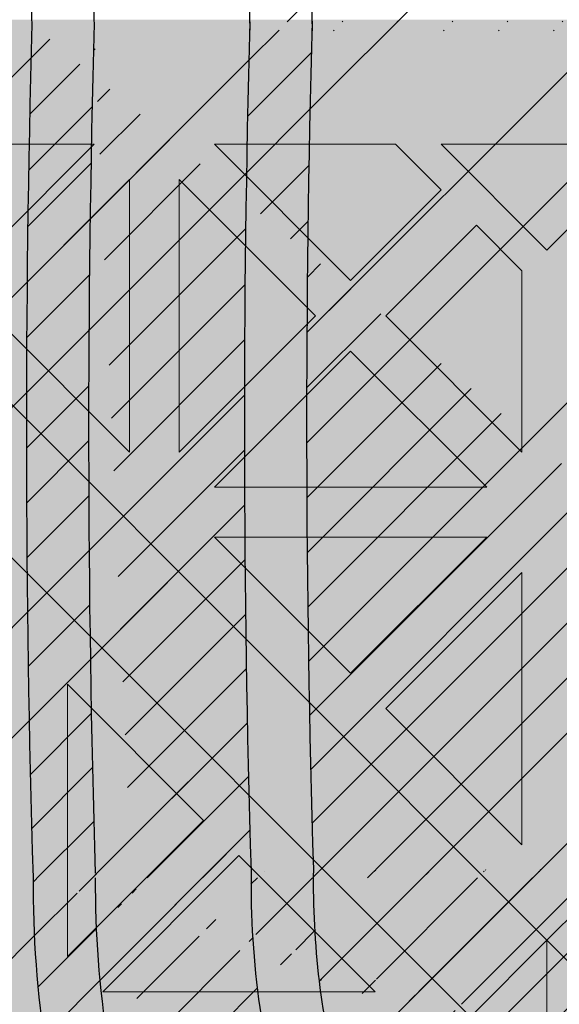
# Model space of a CAD drawing. Units: inches. Extents: x 844 to 2234, y 346 to 1084.
# Tile 54 of 93: x 1866.641 to 1869.404, y 696.327 to 701.365. Entities that reach past the tile are written whole.
import ezdxf

# ---------------------------------------------------------------- set-up
doc = ezdxf.new("R2010")
doc.units = ezdxf.units.IN
doc.header["$MEASUREMENT"] = 0
doc.layers.add('furniture', color=8, linetype='Continuous', lineweight=18)
doc.layers.add('RA-AP-01$0$INT', color=35, linetype='Continuous', lineweight=5)
doc.layers.add('RA-AP-01$0$FURN', color=3, linetype='Continuous')
doc.layers.add('RA-AP-01$0$WOOD', color=64, linetype='Continuous')

# ---------------------------------------------------------------- blocks, each defined once
blk = doc.blocks.new('A$C18D01794')
at = {"layer": 'RA-AP-01$0$INT'}
h = blk.add_hatch(color=256, dxfattribs=at)
h.paths.add_polyline_path([(4.585917135068449, -6.356712009588271), (4.555206456959269, -6.35671200958746), (4.555206456959137, -6.387422687716308), (4.874495778835233, -6.706712009592356), (4.90520645695423, -6.676001331474049)])
h.paths.add_polyline_path([(5.255206456948813, -6.387422687716306), (5.255206456948682, -6.356712009605972), (5.224495778822613, -6.356712009605161), (4.905206456953498, -6.676001331474273), (4.935917135072151, -6.706712009592924)])
h.paths.add_polyline_path([(4.935917135072559, -6.706712009592068), (4.905206456953564, -6.737422687710376), (5.255206456951813, -7.087422687708613), (5.255206456951549, -7.026001331471008)])
h.paths.add_polyline_path([(4.555206456956399, -7.026001331471013), (4.555206456956134, -7.087422687708616), (4.905206456953821, -6.737422687710943), (4.874495778835166, -6.70671200959229)])
h = blk.add_hatch(color=256, dxfattribs=at)
h.paths.add_polyline_path([(4.585917135068448, -6.356712009588273), (4.614201406330596, -6.356712009589021), (4.668846067270487, -6.411356670531338), (4.723490728212344, -6.356712009591912), (4.771774999457151, -6.35671200959319), (4.826419660396886, -6.411356670535356), (4.862780050090322, -6.374996280843536), (4.844495778842715, -6.356712009595112), (4.862780050090411, -6.356712009595595), (4.905206456960182, -6.399138416468211), (4.947632863832445, -6.356712009597838), (4.965917135079675, -6.356712009598322), (4.947632863831759, -6.374996280845421), (4.983993253523576, -6.411356670538857), (5.038637914464627, -6.356712009600247), (5.08692218571208, -6.356712009601523), (5.141566846649976, -6.411356670541852), (5.196211507589851, -6.356712009604411), (5.224495778822615, -6.356712009605161), (4.905206456953975, -6.676001331473793)])
h.paths.add_polyline_path([(4.895206456956031, -6.637717060225675), (4.895206456958921, -6.528427738347902), (4.840561796018589, -6.583072399285802)], flags=16)
h.paths.add_polyline_path([(4.915206456955638, -6.637717060226121), (4.969851117895509, -6.583072399288678), (4.915206456957609, -6.528427738348344)], flags=16)
h.paths.add_polyline_path([(4.826419660395175, -6.568930263661755), (4.881064321335613, -6.514285602723745), (4.771774999456703, -6.514285602720857)], flags=16)
h.paths.add_polyline_path([(4.983993253519558, -6.568930263665262), (5.038637914460456, -6.514285602726792), (4.929348592581548, -6.514285602724816)], flags=16)
h.paths.add_polyline_path([(4.881064321336025, -6.494285602723742), (4.826419660397532, -6.439640941782821), (4.771774999457062, -6.494285602720859)], flags=16)
h.paths.add_polyline_path([(4.929348592582019, -6.494285602724817), (5.038637914460982, -6.494285602726792), (4.983993253522945, -6.439640941786327)], flags=16)
h.paths.add_polyline_path([(4.895206456960191, -6.480143467100443), (4.895206456962115, -6.407422687715913), (4.876922185715016, -6.389138416467584), (4.840561796021581, -6.425498806159401)], flags=16)
h.paths.add_polyline_path([(4.915206456958487, -6.480143467100889), (4.969851117899527, -6.425498806162279), (4.933490728206909, -6.389138416468043), (4.9152064569598, -6.40742268771434)], flags=16)
h.paths.add_polyline_path([(4.757632863832376, -6.480143467096812), (4.812277524772842, -6.425498806158772), (4.757632863834348, -6.370854145217844)], flags=16)
h.paths.add_polyline_path([(4.737632863832376, -6.480143467096286), (4.737632863834348, -6.370854145217375), (4.682988202893906, -6.425498806155385)], flags=16)
h.paths.add_polyline_path([(5.05278005008503, -6.480143467103376), (5.052780050087917, -6.370854145224413), (4.998135389146995, -6.425498806162908)], flags=16)
h.paths.add_polyline_path([(5.072780050085024, -6.480143467103744), (5.127424711025931, -6.42549880616527), (5.072780050087916, -6.370854145224832)], flags=16)
h.paths.add_polyline_path([(4.935917135072783, -6.706712009592292), (5.255206456948811, -6.387422687716309), (5.255206456948932, -6.415706958964177), (5.200561796010279, -6.470351619902839), (5.255206456949403, -6.524996280841948), (5.25520645694961, -6.5732805520894), (5.200561796009787, -6.627925213029239), (5.236922185702417, -6.664285602721864), (5.255206456949919, -6.646001331474357), (5.255206456949998, -6.664285602721898), (5.212780050078687, -6.706712009592262), (5.25520645695036, -6.749138416463932), (5.255206456950438, -6.767422687711313), (5.236922185702424, -6.749138416463297), (5.200561796009796, -6.785498806155928), (5.255206456950753, -6.840143467096874), (5.25520645695096, -6.888427738341682), (5.200561796010322, -6.943072399282328), (5.255206456951428, -6.997717060223427), (5.255206456951547, -7.026001331471006)])
h.paths.add_polyline_path([(5.042988202883395, -6.785498806155427), (5.097632863823085, -6.840143467095101), (5.097632863822622, -6.730854145216193)], flags=16)
h.paths.add_polyline_path([(5.028846067259663, -6.771356670531693), (5.083490728198774, -6.716712009592573), (4.974201406321001, -6.716712009593042)], flags=16)
h.paths.add_polyline_path([(5.117632863823087, -6.840143467095186), (5.172277524762331, -6.785498806155926), (5.11763286382262, -6.730854145216225)], flags=16)
h.paths.add_polyline_path([(5.08349072819877, -6.696712009593886), (5.028846067259652, -6.642067348654775), (4.974201406320998, -6.696712009593438)], flags=16)
h.paths.add_polyline_path([(5.131774999446817, -6.854285602718917), (5.186419660386065, -6.799640941779662), (5.241064321325782, -6.854285602719365)], flags=17)
h.paths.add_polyline_path([(5.131774999446228, -6.716712009592374), (5.186419660386065, -6.771356670532194), (5.222780050079488, -6.734996280838764), (5.204495778832781, -6.716712009592063)], flags=16)
h.paths.add_polyline_path([(5.097632863822613, -6.682569873970264), (5.097632863823061, -6.573280552091354), (5.042988202883383, -6.627925213031044)], flags=16)
h.paths.add_polyline_path([(5.131774999446899, -6.874285602718915), (5.241064321325809, -6.874285602719364), (5.186419660386591, -6.928930263658598)], flags=17)
h.paths.add_polyline_path([(5.131774999446226, -6.696712009594078), (5.204495778830767, -6.696712009594374), (5.22278005007868, -6.67842773834687), (5.186419660386049, -6.642067348654249)], flags=16)
h.paths.add_polyline_path([(5.11763286382262, -6.682569873970225), (5.17227752476232, -6.627925213030515), (5.117632863823064, -6.573280552091267)], flags=16)
h.paths.add_polyline_path([(5.186419660386069, -6.613783077405491), (5.241064321325754, -6.559138416465795), (5.131774999446791, -6.559138416466263)], flags=16)
h.paths.add_polyline_path([(5.131774999446872, -6.539138416466263), (5.24106432132578, -6.539138416465794), (5.186419660386554, -6.484493755526573)], flags=16)
h.paths.add_polyline_path([(5.255206456951811, -7.08742268770861), (5.255206456951895, -7.106712009588038), (4.555206456956052, -7.106712009588038), (4.555206456956136, -7.087422687708617), (4.905206456953973, -6.737422687710788)])
h.paths.add_polyline_path([(4.983993253513404, -6.8444937555241), (4.92934859257295, -6.899138416462108), (5.03863791445186, -6.899138416465014)], flags=16)
h.paths.add_polyline_path([(4.969851117889988, -6.83035161990006), (4.915206456952556, -6.775706958960171), (4.915206456949648, -6.884996280837944)], flags=16)
h.paths.add_polyline_path([(4.929348592572535, -6.919138416462105), (4.983993253511019, -6.973783077403037), (5.038637914451496, -6.919138416465012)], flags=16)
h.paths.add_polyline_path([(5.052780050074912, -6.93328055208906), (4.998135389134438, -6.987925213027088), (5.052780050072919, -7.042569873968025)], flags=16)
h.paths.add_polyline_path([(5.07278005007491, -6.933280552089588), (5.072780050072918, -7.042569873968497), (5.127424711013374, -6.987925213030498)], flags=16)
h.paths.add_polyline_path([(4.89520645695295, -6.775706958959721), (4.840561796013067, -6.830351619897157), (4.895206456950961, -6.884996280837494)], flags=16)
h.paths.add_polyline_path([(4.915206456948365, -6.933280552085403), (4.915206456946434, -7.006001331471951), (4.933490728192729, -7.024285602719066), (4.969851117886972, -6.987925213026453)], flags=16)
h.paths.add_polyline_path([(4.881064321327021, -6.899138416461022), (4.82641966038902, -6.84449375552057), (4.771774999448108, -6.899138416459029)], flags=16)
h.paths.add_polyline_path([(4.895206456950073, -6.933280552084951), (4.840561796009022, -6.987925213023558), (4.876922185700835, -7.024285602716997), (4.895206456948749, -7.006001331469487)], flags=16)
h.paths.add_polyline_path([(4.983993253510392, -7.0020673486505), (4.947632863816944, -7.038427738342319), (4.965917135064043, -7.05671200959023), (5.038637914448995, -7.056712009591555)], flags=16)
h.paths.add_polyline_path([(4.881064321326543, -6.91913841646102), (4.771774999447578, -6.919138416459031), (4.826419660385607, -6.973783077399508)], flags=16)
h.paths.add_polyline_path([(4.905206456946447, -7.014285602717636), (4.862780050074785, -7.056712009588352), (4.947632863816685, -7.056712009589775)], flags=16)
h.paths.add_polyline_path([(5.14156684663679, -7.002067348654549), (5.086922185696452, -7.056712009592438), (5.196211507574223, -7.056712009594425)], flags=16)
h.paths.add_polyline_path([(4.8264196603837, -7.002067348646972), (4.771774999442643, -7.056712009585575), (4.8444957788276, -7.056712009587508), (4.862780050075511, -7.038427738340416)], flags=16)
h.paths.add_polyline_path([(4.812277524760289, -6.98792521302292), (4.757632863822258, -6.933280552082447), (4.757632863819352, -7.042569873961408)], flags=16)
h.paths.add_polyline_path([(4.73763286382226, -6.933280552082079), (4.682988202881349, -6.987925213020536), (4.737632863819352, -7.04256987396099)], flags=16)
h.paths.add_polyline_path([(4.723490728195188, -7.056712009584289), (4.668846067257299, -7.002067348643949), (4.614201406317417, -7.056712009581383)], flags=16)
h.paths.add_polyline_path([(4.597632863829262, -6.706712009592262), (4.555206456957951, -6.664285602721896), (4.555206456958029, -6.646001331474357), (4.573490728205535, -6.664285602721864), (4.609851117898167, -6.627925213029238), (4.555206456958338, -6.573280552089402), (4.555206456958546, -6.524996280841952), (4.60985111789767, -6.470351619902839), (4.555206456959015, -6.415706958964177), (4.555206456959138, -6.387422687716309), (4.874495778835167, -6.70671200959229), (4.5552064569564, -7.026001331471015), (4.555206456956523, -6.997717060223433), (4.609851117897629, -6.94307239928233), (4.555206456956988, -6.888427738341681), (4.555206456957198, -6.840143467096881), (4.609851117898153, -6.78549880615593), (4.573490728205528, -6.749138416463297), (4.555206456957507, -6.76742268771132), (4.555206456957585, -6.749138416463933)])
h.paths.add_polyline_path([(4.712780050085332, -6.730854145216195), (4.712780050084863, -6.840143467095105), (4.767424711024555, -6.785498806155427)], flags=16)
h.paths.add_polyline_path([(4.726922185709173, -6.716712009592573), (4.781566846648288, -6.771356670531693), (4.836211507586949, -6.716712009593043)], flags=16)
h.paths.add_polyline_path([(4.692780050085327, -6.730854145216225), (4.638135389145619, -6.785498806155928), (4.692780050084865, -6.840143467095185)], flags=16)
h.paths.add_polyline_path([(4.726922185709182, -6.696712009593886), (4.836211507586949, -6.696712009593436), (4.7815668466483, -6.642067348654773)], flags=16)
h.paths.add_polyline_path([(4.678637914461726, -6.71671200959237), (4.605917135075169, -6.716712009592063), (4.587632863828464, -6.734996280838766), (4.623993253521887, -6.771356670532195)], flags=16)
h.paths.add_polyline_path([(4.712780050085336, -6.68256987397026), (4.767424711024568, -6.627925213031042), (4.71278005008489, -6.573280552091352)], flags=16)
h.paths.add_polyline_path([(4.678637914461726, -6.696712009594076), (4.623993253521899, -6.642067348654247), (4.587632863829271, -6.67842773834687), (4.605917135077185, -6.696712009594376)], flags=16)
h.paths.add_polyline_path([(4.692780050085336, -6.682569873970228), (4.692780050084889, -6.573280552091267), (4.638135389145632, -6.627925213030515)], flags=16)
h.paths.add_polyline_path([(4.623993253521885, -6.799640941779662), (4.678637914461131, -6.854285602718915), (4.56934859258217, -6.854285602719365)], flags=17)
h.paths.add_polyline_path([(4.623993253521901, -6.613783077405509), (4.678637914461158, -6.559138416466263), (4.569348592582195, -6.559138416465795)], flags=16)
h.paths.add_polyline_path([(4.678637914461051, -6.874285602718915), (4.623993253521361, -6.928930263658598), (4.569348592582143, -6.874285602719364)], flags=17)
h.paths.add_polyline_path([(4.678637914461076, -6.539138416466263), (4.623993253521399, -6.484493755526573), (4.569348592582167, -6.539138416465796)], flags=16)
h = blk.add_hatch(color=256, dxfattribs=at)
h.paths.add_polyline_path([(4.781566846647504, -6.771356670530272), (4.836211507586161, -6.716712009591613), (4.726922185708388, -6.716712009591159)])
h.paths.add_polyline_path([(4.836211507586161, -6.696712009592008), (4.781566846647504, -6.642067348653354), (4.726922185708388, -6.69671200959247)])
h.paths.add_polyline_path([(4.76742471102377, -6.627925213029623), (4.712780050084083, -6.57328055208994), (4.712780050084542, -6.68256987396885)])
h.paths.add_polyline_path([(4.692780050084544, -6.682569873968819), (4.692780050084084, -6.573280552089856), (4.638135389144834, -6.627925213029111)])
h.paths.add_polyline_path([(4.678637914460932, -6.696712009592669), (4.623993253521102, -6.642067348652844), (4.587632863827676, -6.678427738346266), (4.605917135074382, -6.696712009592973)])
h.paths.add_polyline_path([(4.573490728204743, -6.664285602721736), (4.60985111789737, -6.627925213029108), (4.555206456957541, -6.573280552089279), (4.555206456957237, -6.646001331474231)])
h.paths.add_polyline_path([(4.623993253521098, -6.613783077405377), (4.67863791446035, -6.559138416466126), (4.56934859258139, -6.559138416465669)])
h.paths.add_polyline_path([(4.678637914460275, -6.539138416466126), (4.623993253520583, -6.48449375552644), (4.56934859258136, -6.539138416465672)])
h.paths.add_polyline_path([(4.609851117896854, -6.470351619902707), (4.555206456958196, -6.415706958964051), (4.555206456957738, -6.524996280841822)])
h.paths.add_polyline_path([(4.597632863828475, -6.706712009592775), (4.555206456957283, -6.664285602721582), (4.555206456956805, -6.749138416463489)])
h.paths.add_polyline_path([(4.678637914460932, -6.716712009590963), (4.605917135076396, -6.71671200959066), (4.587632863828479, -6.734996280838164), (4.623993253521104, -6.771356670530792)])
h.paths.add_polyline_path([(4.692780050084091, -6.840143467093776), (4.692780050084548, -6.730854145214809), (4.638135389144834, -6.785498806154524)])
h.paths.add_polyline_path([(4.767424711023772, -6.785498806154004), (4.712780050084545, -6.730854145214786), (4.712780050084089, -6.840143467093692)])
h.paths.add_polyline_path([(4.67863791446036, -6.854285602718778), (4.623993253521105, -6.799640941779527), (4.569348592581399, -6.854285602719237)])
h.paths.add_polyline_path([(4.609851117897371, -6.785498806155798), (4.573490728204743, -6.74913841646317), (4.555206456957237, -6.767422687710675), (4.555206456957548, -6.840143467095629)])
h.paths.add_polyline_path([(4.623993253520596, -6.928930263658465), (4.67863791446028, -6.874285602718778), (4.569348592581367, -6.874285602719238)])
h.paths.add_polyline_path([(4.609851117896867, -6.943072399282199), (4.555206456957749, -6.888427738343082), (4.55520645695821, -6.997717060220857)])
h = blk.add_hatch(color=256, dxfattribs=at)
h.paths.add_polyline_path([(4.905206456953579, -6.70671200959253), (4.905206456953751, -6.676001331474523), (4.874495778835229, -6.706712009592358)])
h.paths.add_polyline_path([(4.935917135071924, -6.706712009592703), (4.905206456953583, -6.706712009592529), (4.90520645695341, -6.737422687710532)])
h = blk.add_hatch(color=256, dxfattribs=at)
h.paths.add_polyline_path([(4.905206456953409, -6.737422687710532), (4.90520645695358, -6.706712009592529), (4.874495778835235, -6.706712009592359)])
h.paths.add_polyline_path([(4.935917135071928, -6.706712009592703), (4.905206456953754, -6.676001331474527), (4.905206456953582, -6.706712009592529)])
h = blk.add_hatch(color=256, dxfattribs=at)
h.paths.add_polyline_path([(4.895206456952951, -6.77570695895972), (4.840561796013068, -6.830351619897156), (4.895206456950958, -6.884996280837495)])
h.paths.add_polyline_path([(4.915206456949649, -6.884996280837942), (4.969851117889987, -6.830351619900054), (4.915206456952556, -6.775706958960171)])
h.paths.add_polyline_path([(5.038637914451862, -6.899138416465013), (4.983993253513403, -6.8444937555241), (4.929348592572953, -6.899138416462106)])
h.paths.add_polyline_path([(4.929348592572535, -6.919138416462105), (4.983993253511018, -6.973783077403037), (5.038637914451497, -6.919138416465012)])
h.paths.add_polyline_path([(4.915206456948366, -6.933280552085397), (4.915206456946433, -7.006001331471951), (4.93349072819273, -7.024285602719068), (4.969851117886972, -6.987925213026454)])
h.paths.add_polyline_path([(5.038637914448995, -7.056712009591553), (4.983993253510389, -7.002067348650502), (4.947632863816946, -7.038427738342318), (4.965917135064043, -7.05671200959023)])
h.paths.add_polyline_path([(5.05278005007292, -7.042569873968023), (5.05278005007491, -6.933280552089059), (4.998135389134438, -6.987925213027088)])
h.paths.add_polyline_path([(5.07278005007292, -7.042569873968496), (5.127424711013374, -6.987925213030498), (5.072780050074909, -6.933280552089588)])
h.paths.add_polyline_path([(5.141566846636789, -7.002067348654547), (5.086922185696449, -7.056712009592438), (5.196211507574223, -7.056712009594425)])
h.paths.add_polyline_path([(4.947632863816688, -7.056712009589774), (4.905206456946449, -7.014285602717634), (4.862780050074784, -7.056712009588353)])
h.paths.add_polyline_path([(4.840561796009025, -6.987925213023556), (4.876922185700834, -7.024285602716997), (4.895206456948747, -7.006001331469488), (4.895206456950075, -6.933280552084953)])
h.paths.add_polyline_path([(4.88106432132654, -6.919138416461021), (4.771774999447577, -6.919138416459031), (4.826419660385606, -6.973783077399508)])
h.paths.add_polyline_path([(4.881064321327019, -6.899138416461022), (4.826419660389019, -6.844493755520571), (4.771774999448108, -6.89913841645903)])
h.paths.add_polyline_path([(4.757632863819352, -7.042569873961409), (4.812277524760284, -6.987925213022922), (4.757632863822259, -6.933280552082447)])
h.paths.add_polyline_path([(4.8264196603837, -7.002067348646974), (4.771774999442646, -7.056712009585575), (4.844495778827599, -7.05671200958751), (4.862780050075512, -7.038427738340417)])
h.paths.add_polyline_path([(4.737632863819352, -7.042569873960988), (4.737632863822258, -6.933280552082078), (4.682988202881349, -6.987925213020538)])
h.paths.add_polyline_path([(4.668846067257299, -7.002067348643952), (4.61420140631742, -7.056712009581384), (4.723490728195189, -7.056712009584292)])
for p, q in [((4.905206456953753, -6.676001331474525), (4.905206456953409, -6.737422687710532)), ((4.874495778835167, -6.70671200959229), (4.555206456956399, -7.026001331471013)), ((4.874495778835233, -6.706712009592356), (4.905206456953409, -6.737422687710532)), ((4.935917135071927, -6.706712009592701), (4.905206456953407, -6.737422687710532)), ((4.726922185709178, -6.716712009592574), (4.836211507586949, -6.716712009593042)), ((4.72692218570918, -6.716712009592578), (4.781566846648288, -6.771356670531693)), ((4.836211507586949, -6.716712009593042), (4.781566846648288, -6.771356670531693)), ((4.712780050084865, -6.840143467095105), (4.71278005008533, -6.730854145216195)), ((4.71278005008533, -6.730854145216195), (4.767424711024555, -6.785498806155425)), ((4.905206456953975, -6.737422687710788), (4.555206456956136, -7.087422687708617)), ((4.905206456953975, -6.737422687710788), (5.255206456951811, -7.087422687708611)), ((4.89520645695295, -6.775706958959723), (4.840561796013068, -6.830351619897156)), ((4.895206456950959, -6.884996280837494), (4.89520645695295, -6.775706958959723)), ((4.767424711024554, -6.785498806155427), (4.712780050084865, -6.840143467095105)), ((4.895206456950956, -6.884996280837492), (4.840561796013068, -6.830351619897156)), ((4.826419660389018, -6.844493755520574), (4.771774999448109, -6.899138416459031)), ((4.881064321327019, -6.899138416461022), (4.82641966038902, -6.844493755520572)), ((4.771774999448109, -6.899138416459031), (4.881064321327019, -6.899138416461022)), ((4.771774999447578, -6.919138416459031), (4.881064321326541, -6.919138416461022)), ((4.771774999447578, -6.919138416459031), (4.826419660385606, -6.973783077399508)), ((4.881064321326541, -6.919138416461022), (4.826419660385606, -6.973783077399508)), ((4.682988202881351, -6.987925213020536), (4.737632863822258, -6.933280552082079)), ((4.737632863822258, -6.933280552082079), (4.737632863819352, -7.042569873960989)), ((4.757632863822258, -6.933280552082445), (4.812277524760285, -6.987925213022922)), ((4.757632863822258, -6.933280552082445), (4.757632863819352, -7.042569873961408)), ((4.895206456950073, -6.933280552084951), (4.840561796009024, -6.987925213023556)), ((4.895206456948748, -7.006001331469903), (4.895206456950073, -6.933280552084951)), ((4.737632863819352, -7.042569873960989), (4.682988202881349, -6.987925213020538)), ((4.757632863819352, -7.042569873961408), (4.812277524760285, -6.987925213022922)), ((4.840561796009024, -6.987925213023554), (4.876922185700835, -7.024285602716997)), ((4.723490728195186, -7.056712009584289), (4.668846067257299, -7.002067348643951)), ((4.771774999442645, -7.056712009585574), (4.8264196603837, -7.002067348646972)), ((4.826419660383698, -7.002067348646972), (4.862780050075511, -7.038427738340416)), ((4.895206456946431, -7.006001331471805), (4.876922185700835, -7.024285602716997)), ((4.905206456946449, -7.014285602717635), (4.862780050074783, -7.056712009588354)), ((4.905206456946449, -7.014285602717635), (4.94763286381669, -7.056712009589775)), ((4.844495778827597, -7.056712009587512), (4.862780050075513, -7.038427738340416)), ((4.723490728195188, -7.056712009584293), (4.614201406317417, -7.056712009581383)), ((4.844495778827597, -7.05671200958751), (4.771774999442645, -7.056712009585574)), ((4.94763286381669, -7.056712009589775), (4.862780050074783, -7.056712009588354))]:
    blk.add_line(p, q, dxfattribs=at)
blk = doc.blocks.new('A$C32926AE1')
at = {"layer": 'RA-AP-01$0$FURN'}
h = blk.add_hatch(dxfattribs=at)
h.set_pattern_fill('ANSI31', color=256, scale=0.1, style=0)
h.set_pattern_definition([(45, (0, 0), (-0.0088388347648318, 0.0088388347648318), [])])
edge = h.paths.add_edge_path(flags=16)
edge.add_arc((4.904771284329206, 4.246793130718756), 0.2603971832811541, 75.22398030683196, 104.7760196931204)
edge.add_arc((4.904771284329206, 4.246793130718756), 0.2603971832811541, 75.223980306832, 104.77601969312039, ccw=False)
edge = h.paths.add_edge_path(flags=16)
edge.add_arc((4.904771284329206, 4.067062675376612), 0.2603971832811541, 255.2239803068796, 284.776019693168)
edge.add_arc((4.904771284329206, 4.067062675376612), 0.2603971832811541, 255.22398030687958, 284.77601969316805, ccw=False)
edge = h.paths.add_edge_path(flags=0)
edge.add_arc((4.904771284329206, 4.067062675376612), 0.2603971832811541, 255.2239803068796, 284.776019693168)
edge.add_arc((4.904771284329206, 4.067062675376612), 0.2603971832811541, 255.22398030687958, 284.77601969316805, ccw=False)
edge = h.paths.add_edge_path(flags=0)
edge.add_arc((4.904771284329206, 4.067062675376612), 0.2603971832811541, 255.2239803068796, 284.776019693168)
edge.add_arc((4.904771284329206, 4.067062675376612), 0.2603971832811541, 255.22398030687958, 284.77601969316805, ccw=False)
edge = h.paths.add_edge_path()
edge.add_arc((4.604388392048174, 4.588829985554312), 0.1599999999999918, 342.3781640246255, 354.4317409793762)
edge.add_arc((5.090145208887507, 4.43216705527679), 0.3503971832811637, 162.0091218307731, 180.3186872093483)
edge.add_arc((5.205154176610243, 4.588829985554953), 0.1599999999999917, 185.5682590208461, 197.6218359767349)
edge.add_arc((4.904771284329229, 4.246793130718735), 0.3503971832811761, 72.00912183053516, 107.9908781690354)
edge.add_arc((9.535952835716557, 4.28682295566602), 4.798342501046485, 178.2875002453811, 181.5576802719453)
edge.add_arc((4.719397359771122, 4.43216705527679), 0.3503971832811637, 359.6813127906516, 377.9908781692269)
edge.add_arc((9.535967292294904, 4.286822350292874), 4.778371420254705, 178.2965938931842, 181.5667745797229)
edge.add_arc((4.719397359771122, 4.43216705527679), 0.3303971832811637, 359.6813127906516, 377.9908781692269)
edge.add_arc((0.2735752763637294, 4.286822350292874), 4.7783714202547, 358.4332254202771, 361.7034061068158)
edge.add_arc((5.061434214606998, 4.732549947558029), 0.1600000000000254, 252.3781640250584, 264.4317409792362)
edge.add_arc((4.748108354051257, 4.732549947558012), 0.1600000000000541, 275.5682590208426, 287.6218359759532)
edge.add_arc((4.604388392048115, 4.588829985554317), 0.1800000000000505, 342.3567572500182, 349.3735009646207)
edge.add_arc((5.205154176610254, 4.588829985554976), 0.1800000000000069, 190.6264990356027, 197.6432427513933)
edge.add_arc((5.061434214607106, 4.732549947558013), 0.1800000000000424, 252.3567572496606, 259.3735009644582)
edge.add_arc((4.904771284329208, 4.246793130718737), 0.3303971832811676, 71.99844483668534, 108.0015551637021)
edge.add_arc((4.748108354051414, 4.732549947558045), 0.1800000000000547, 280.6264990355479, 287.6432427495938)
edge.add_arc((5.090145208887514, 4.432167055276789), 0.2803971832811691, 162.8706300666893, 180.816523289902)
edge.add_arc((4.719397359771136, 4.432167055276689), 0.2803971832811534, 359.183476710103, 377.1293699333214)
edge.add_arc((4.904771284329222, 4.246793130718737), 0.2803971832811769, 72.87063006672916, 107.1293699332334)
edge.add_arc((5.090145208887522, 4.432167055276788), 0.2603971832811776, 165.2239803068007, 180.9953123810312)
edge.add_arc((4.719397359771141, 4.432167055276699), 0.2603971832811458, 359.0046876189768, 374.7760196932087)
edge.add_arc((5.090145208887507, 4.43216705527679), 0.3303971832811637, 162.0091218307731, 180.3186872093483)
edge.add_arc((9.53595427642584, 4.285015535491528), 4.728345371032053, 178.265043920078, 181.5679956281801)
edge.add_arc((0.2735882922327999, 4.285015535491582), 4.728345371032045, 358.4320043718193, 361.7349560799204)
edge.add_arc((9.535953591267507, 4.284458026472751), 4.708343996644348, 178.2573054306777, 181.5704995759608)
edge.add_arc((0.273588977391114, 4.284458026472785), 4.708343996644358, 358.4295004240388, 361.7426945693213)
edge.add_arc((0.2735889773911131, 4.029397779622582), 4.708343996644359, 358.2573054306787, 361.5704995759613)
edge.add_arc((9.535953591267518, 4.029397779622618), 4.708343996644359, 178.4295004240391, 181.7426945693223)
edge.add_arc((0.2735882922327901, 4.028840270603786), 4.728345371032054, 358.2650439200796, 361.5679956281808)
edge.add_arc((9.53595427642584, 4.028840270603841), 4.728345371032054, 178.4320043718199, 181.7349560799219)
edge.add_arc((0.2735752763637302, 4.027033455802493), 4.778371420254699, 358.2965938931842, 361.5667745797229)
edge.add_arc((4.719397359771122, 3.881688750818578), 0.3303971832811637, 342.0091218307731, 360.3186872093484)
edge.add_arc((5.090145208887507, 3.881688750818578), 0.3303971832811637, 179.6813127906516, 197.9908781692269)
edge.add_arc((9.535967292294904, 4.027033455802493), 4.778371420254705, 178.433225420277, 181.7034061068158)
edge.add_arc((4.719397359771122, 3.881688750818578), 0.3503971832811637, 342.0091218307731, 360.3186872093484)
edge.add_arc((9.53595283571655, 4.027032850429349), 4.79834250104648, 178.4423197280546, 181.7124997546188)
edge.add_arc((4.719397359771141, 3.881688750818669), 0.2603971832811458, 345.2239803067913, 360.9953123810232)
edge.add_arc((5.090145208887522, 3.88168875081858), 0.2603971832811776, 179.0046876189687, 194.7760196931993)
edge.add_arc((4.904771284329222, 4.067062675376631), 0.2803971832811769, 252.8706300667665, 287.1293699332708)
edge.add_arc((4.719397359771136, 3.881688750818678), 0.2803971832811534, 342.8706300666787, 360.8165232898969)
edge.add_arc((5.090145208887514, 3.881688750818579), 0.2803971832811691, 179.183476710098, 197.1293699333106)
edge.add_arc((4.748108354051414, 3.581305858537323), 0.1800000000000547, 72.3567572504062, 79.37350096445199)
edge.add_arc((4.904771284329208, 4.067062675376631), 0.3303971832811676, 251.9984448362979, 288.0015551633146)
edge.add_arc((5.061434214607106, 3.581305858537355), 0.1800000000000424, 100.6264990355418, 107.6432427503394)
edge.add_arc((5.205154176610254, 3.725025820540392), 0.1800000000000069, 162.3567572486066, 169.3735009643972)
edge.add_arc((4.604388392048115, 3.725025820541051), 0.1800000000000505, 10.62649903537925, 17.64324274998182)
edge.add_arc((4.748108354051257, 3.581305858537356), 0.1600000000000541, 72.37816402404681, 84.43174097915735)
edge.add_arc((4.904771284329229, 4.067062675376632), 0.3503971832811761, 252.0091218309645, 287.9908781694648)
edge.add_arc((5.061434214606998, 3.581305858537339), 0.1600000000000254, 95.56825902076373, 107.6218359749416)
edge.add_arc((5.205154176610243, 3.725025820540414), 0.1599999999999917, 162.3781640232651, 174.4317409791539)
edge.add_arc((5.090145208887507, 3.881688750818578), 0.3503971832811637, 179.6813127906516, 197.9908781692269)
edge.add_arc((4.604388392048174, 3.725025820541056), 0.1599999999999918, 5.568259020623824, 17.62183597537444)
edge.add_arc((0.2735897329420762, 4.28682295566602), 4.798342501046482, 358.4423197280547, 361.7124997546188)
edge.add_arc((0.2735897329420691, 4.027032850429348), 4.798342501046489, 358.2875002453812, 361.5576802719453)
at = {"layer": 'RA-AP-01$0$WOOD'}
h = blk.add_hatch(color=256, dxfattribs=at)
h.dxf.hatch_style = 1
h.paths.add_polyline_path([(5.157430609644524, 4.573483066760929, -0.1009492694046607), (5.155401577623758, 4.593365984175333, -0.1842662638101597), (5.172249623284174, 4.638795604568598, 0.2056608120311276), (5.179560981299304, 4.661316324430096, 0.3614336704623542), (5.134352340494423, 4.706524965234944, 0.2056608120311297), (5.111831620632933, 4.699213607219793, -0.1842662638101113), (5.066402000239693, 4.682365561559342, -0.1055311479399994), (5.045656153913092, 4.68467289944697, 0.1567636581983829), (4.763886414745334, 4.684672899446966, -0.1055311479399895), (4.743140568418733, 4.68236556155934, -0.1842662638100833), (4.6977109480255, 4.69921360721979, 0.2056608120302612), (4.675190228164109, 4.706524965234949, 0.3614336704708441), (4.629981587358889, 4.66131632442871, 0.2056608120245944), (4.637292945374126, 4.638795604567974, -0.1842662638101024), (4.654140991034615, 4.59336598417475, -0.1009492694055169), (4.652111959013835, 4.573483066760181, 0.021410119221476), (4.629748025606143, 4.156712009541676, 0.0214101192214795), (4.652111959013809, 3.739940952323101, -0.1009492694059586), (4.654140991034615, 3.720058034908448, -0.1842662638100975), (4.637292945374126, 3.674628414515226, 0.2056608120245705), (4.629981587358889, 3.652107694654492, 0.3614336704708879), (4.675190228164113, 3.606899053848249, 0.2056608120302384), (4.697710948025501, 3.614210411863408, -0.1842662638100995), (4.743140568418738, 3.63105845752386, -0.1055311479402541), (4.763886414745388, 3.628751119636215, 0.1567636581983776), (5.045656153913137, 3.628751119636244, -0.1055311479397538), (5.066402000239692, 3.631058457523857, -0.1842662638101067), (5.111831620632931, 3.614210411863407, 0.2056608120310924), (5.134352340494417, 3.606899053848256, 0.3614336704624001), (5.179560981299307, 3.652107694653103, 0.2056608120311314), (5.172249623284175, 3.6746284145146, -0.1842662638101402), (5.155401577623758, 3.72005803490786, -0.1009492694051366), (5.15743060964455, 3.739940952322354, 0.0214101192215073), (5.179794543052287, 4.156712009541468, 0.0214101192215252)])
h.paths.add_polyline_path([(4.639748609479751, 4.156712009541513, 0.0213537860821624), (4.661970494867118, 3.741887061152232, -0.094075836301374), (4.664143710413708, 3.7196126951003, -0.1824818158568985), (4.644813765429836, 3.668037719127816, 0.2056608120245319), (4.639939526753007, 3.653023905887301, 0.3614336704710246), (4.676106439397173, 3.616856993242342, 0.2056608120302234), (4.691120252638095, 3.621731231919122, -0.1824818158602558), (4.742695228611606, 3.641061176902986, -0.1029891339458722), (4.766991894714349, 3.638256818950944, 0.156709409989566), (5.042550673941472, 3.638256818950105, -0.102989133958497), (5.066847340047078, 3.641061176902949, -0.1824818158594995), (5.118422316020358, 3.621731231919103, 0.2056608120311416), (5.133436129261316, 3.616856993242346, 0.3614336704621468), (5.169603041905217, 3.653023905886178, 0.2056608120310986), (5.164728803228477, 3.668037719127177, -0.1824818158565612), (5.145398858244737, 3.719612695099578, -0.0940758363009313), (5.147572073791232, 3.741887061151398, 0.0213537860822023), (5.169793959178681, 4.156712009541451, 0.0213537860822226), (5.147572073791203, 4.571536957931898, -0.0940758363005034), (5.145398858244737, 4.59381132398362, -0.1824818158565587), (5.164728803228476, 4.645386299956021, 0.2056608120311045), (5.169603041905216, 4.66040011319702, 0.3614336704621845), (5.133436129261313, 4.696567025840856, 0.2056608120310773), (5.118422316020359, 4.691692787164098, -0.182481815859508), (5.066847340047078, 4.67236284218025, -0.1029891339584606), (5.04255067394148, 4.675167200133092, 0.156709409989566), (4.766991894714357, 4.675167200132257, -0.1029891339458842), (4.742695228611611, 4.672362842180213, -0.1824818158602725), (4.691120252638095, 4.691692787164077, 0.2056608120302152), (4.676106439397174, 4.696567025840858, 0.3614336704710363), (4.639939526753005, 4.660400113195899, 0.2056608120245495), (4.644813765429837, 4.645386299955384, -0.1824818158568934), (4.664143710413708, 4.593811323982902, -0.0940758363009187), (4.661970494867149, 4.571536957931074, 0.021353786082177)], flags=16)
h.paths.add_polyline_path([(5.129794543052235, 4.432167055276933, -0.0141661062790638), (5.130152669293814, 4.156927903047693, -0.0141661062790647), (5.129794543052234, 3.881688750818433, -0.0785247771143638), (5.10979738006795, 3.755143611847103, 0.0945969212073497), (5.105408519571111, 3.717898134952927, 0.1043170707844957), (5.116074640131521, 3.670385395016088, 0.1043170707864965), (5.068561900193738, 3.681051515576561, 0.09459692119553), (5.031316423304057, 3.676662655080835, -0.1580239521427272), (4.778226145355827, 3.676662655080367, 0.0945969211986668), (4.740980668464973, 3.681051515576592, 0.1043170707882822), (4.693467928526415, 3.670385395015844, 0.1043170707867916), (4.704134049087309, 3.717898134953662, 0.0945969211972894), (4.69974518859162, 3.755143611844042, -0.0785247771163196), (4.679748025606343, 3.881688750818406, -0.0141661062790663), (4.679389899364763, 4.156927903047693, -0.0141661062790672), (4.679748025606343, 4.432167055276998, -0.0785247771163064), (4.699745188591625, 4.55871219425134, 0.094596921197333), (4.704134049087308, 4.595957671141738, 0.1043170707867205), (4.693467928526416, 4.643470411079523, 0.1043170707882628), (4.740980668464965, 4.632804290518776, 0.0945969211988114), (4.778226145355874, 4.637193151015016, -0.158023952142669), (5.031316423304015, 4.637193151014546, 0.0945969211956361), (5.068561900193736, 4.632804290518806, 0.1043170707864979), (5.11607464013152, 4.643470411079278, 0.1043170707844617), (5.105408519571112, 4.595957671142455, 0.0945969212074597), (5.109797380067959, 4.558712194248236, -0.0785247771143467)], flags=0)
h.paths.add_polyline_path([(5.119794532311105, 4.432259799204851, -0.0142000800617244), (5.120156169157484, 4.156927903047701, -0.0142000800617277), (5.119794532311105, 3.881596006890482, -0.0784894509520253), (5.100273383573699, 3.758192358677797, 0.0940138827242913), (5.095413455884425, 3.717477693979438, 0.0606271852308753), (5.099615656341024, 3.686844378806616, 0.0606271852322524), (5.068982341167493, 3.691046579263239, 0.0940138827010453), (5.028267676478798, 3.686186651576848, -0.1580706864508061), (4.781274892180912, 3.686186651576435, 0.0940138827026903), (4.740560227491556, 3.691046579263279, 0.0606271852339895), (4.709926912317155, 3.686844378806508, 0.0606271852329405), (4.714129112773991, 3.717477693980356, 0.094013882701304), (4.709269185087677, 3.758192358669163, -0.0784894509577193), (4.689748036347473, 3.881596006890469, -0.014200080061729), (4.689386399501094, 4.156927903047709, -0.0142000800617217), (4.689748036347473, 4.432259799204808, -0.078489450957724), (4.709269185087651, 4.555663447426125, 0.0940138827014585), (4.714129112773992, 4.596378112114996, 0.0606271852329731), (4.709926912317154, 4.62701142728886, 0.0606271852340196), (4.74056022749157, 4.622809226832087, 0.0940138827024997), (4.781274892180847, 4.627669154518912, -0.1580706864508359), (5.028267676478777, 4.627669154518526, 0.0940138827010946), (5.068982341167492, 4.622809226832129, 0.060627185232254), (5.099615656341024, 4.627011427288751, 0.0606271852308727), (5.095413455884425, 4.59637811211593, 0.0940138827241088), (5.100273383573675, 4.555663447417647, -0.0784894509520978)], flags=0)
h.paths.add_polyline_path([(5.06978912287499, 4.430218106756144, -0.014241683694547), (5.070173729147532, 4.156927903047672, -0.0142416836945458), (5.06978912287499, 3.883637699339223, -0.0800609523125196), (5.052662118612511, 3.773463122773442, 0.0526421978001116), (5.04590916754064, 3.740550867606997, 0.0526421977992423), (5.012996912374707, 3.73379791653534, -0.1583028414718258), (4.796545656286308, 3.73379791653451, 0.0526421978034211), (4.763633401117837, 3.740550867607021, 0.0526421978018622), (4.756880450045755, 3.773463122774558, -0.0800609523117106), (4.739753445783639, 3.883637699339268, -0.0142416836945435), (4.739368839511098, 4.156927903047671, -0.0142416836945477), (4.739753445783639, 4.430218106756155, -0.0800609523116345), (4.75688045004574, 4.540392683320762, 0.052642197801941), (4.763633401117837, 4.573304938488346, 0.0526421978035071), (4.796545656286361, 4.580057889560873, -0.1583028414717561), (5.012996912374669, 4.580057889560039, 0.0526421977993048), (5.04590916754064, 4.57330493848837, 0.0526421978002057), (5.052662118612529, 4.540392683321868, -0.080060952312477)], flags=0)
h.paths.add_polyline_path([(5.049789715110557, 4.43038092723357, -0.0143097550741839), (5.05018085590259, 4.156927903047715, -0.0143097550741854), (5.049789715110558, 3.883474878861827, -0.0800685599149176), (5.03362098255317, 3.779581877367999, 0.0306258898956367), (5.028241146483733, 3.758218888663947, 0.0306258898977031), (5.006878157778253, 3.75283905259408, -0.1583983521624096), (4.802664410878162, 3.752839052594731, 0.0306258898946014), (4.781301422174808, 3.758218888663924, 0.0306258898967912), (4.775921586105202, 3.779581877368794, -0.080068559914251), (4.759752853548071, 3.883474878861786, -0.0143097550741854), (4.759361712756037, 4.156927903047671, -0.0143097550741854), (4.759752853548071, 4.430380927233557, -0.0800685599142479), (4.775921586105193, 4.534273928726546, 0.0306258898968306), (4.781301422174808, 4.555636917431444, 0.0306258898945754), (4.802664410878143, 4.561016753500631, -0.1583983521624168), (5.006878157778244, 4.561016753501291, 0.0306258898977177), (5.028241146483733, 4.555636917431421, 0.0306258898958182), (5.03362098255321, 4.534273928727244, -0.080068559914796)], flags=0)
h.paths.add_polyline_path([(4.999766070382627, 4.428171244713864, -0.0143443147609634), (5.000198441819402, 4.156927903047689, -0.0143443147609612), (4.999766070382627, 3.885684561381556, -0.0784641635803329), (4.987356730658798, 3.799103304488872, -0.1506053783831347), (4.822185837999821, 3.79910330448882, -0.0784641635803318), (4.809776498276007, 3.885684561381509, -0.014344314760963), (4.809344126839227, 4.156927903047677, -0.0143443147609645), (4.809776498276007, 4.428171244713873, -0.0784641635803192), (4.822185837999822, 4.514752501606549, -0.1506053783831338), (4.987356730658798, 4.514752501606494, -0.078464163580285)], flags=0)
h.paths.add_polyline_path([(4.979755254238824, 4.42764379880488, -0.0143772539198268), (4.980205517789977, 4.156927903047693, -0.0143772539198275), (4.979755254238824, 3.886212007290489, -0.0689242507424422), (4.971183264704897, 3.815276770442801, -0.1296645318904179), (4.838359303953726, 3.815276770442746, -0.0689242507424186), (4.829787314419809, 3.886212007290419, -0.0143772539198292), (4.829337050868653, 4.156927903047653, -0.0143772539198325), (4.829787314419809, 4.427643798804946, -0.0689242507424211), (4.838359303953725, 4.498579035652621, -0.1296645318904187), (4.971183264704897, 4.498579035652565, -0.0689242507424401)], flags=0)
h = blk.add_hatch(color=256, dxfattribs=at)
h.dxf.hatch_style = 1
h.paths.add_polyline_path([(5.145398858244737, 4.59381132398362, -0.1824818158565616), (5.164728803228476, 4.645386299956021, 0.2056608120311045), (5.169603041905216, 4.66040011319702, 0.3614336704621845), (5.133436129261313, 4.696567025840856, 0.2056608120310773), (5.118422316020359, 4.691692787164098, -0.182481815859508), (5.066847340047078, 4.67236284218025, -0.1029891339584606), (5.04255067394148, 4.675167200133092, 0.156709409989566), (4.766991894714357, 4.675167200132257, -0.1029891339458842), (4.742695228611611, 4.672362842180213, -0.1824818158602725), (4.691120252638095, 4.691692787164077, 0.2056608120302152), (4.676106439397174, 4.696567025840858, 0.3614336704710363), (4.639939526753005, 4.660400113195899, 0.2056608120245495), (4.644813765429837, 4.645386299955384, -0.1824818158568934), (4.664143710413708, 4.593811323982902, -0.0940758363009187), (4.661970494867149, 4.571536957931074, 0.0213537860821772), (4.639748609479751, 4.156712009541507, 0.0213537860821625), (4.661970494867119, 3.741887061152226, -0.0940758363013071), (4.664143710413708, 3.719612695100309, -0.1824818158569294), (4.644813765429836, 3.668037719127816, 0.2056608120245319), (4.639939526753007, 3.653023905887301, 0.3614336704710246), (4.676106439397173, 3.616856993242342, 0.2056608120302234), (4.691120252638095, 3.621731231919122, -0.1824818158602558), (4.742695228611606, 3.641061176902986, -0.1029891339458722), (4.766991894714349, 3.638256818950944, 0.156709409989566), (5.042550673941472, 3.638256818950105, -0.102989133958497), (5.066847340047078, 3.641061176902949, -0.1824818158594995), (5.118422316020358, 3.621731231919103, 0.2056608120311416), (5.133436129261316, 3.616856993242346, 0.3614336704621468), (5.169603041905217, 3.653023905886178, 0.2056608120310986), (5.164728803228477, 3.668037719127177, -0.1824818158565612), (5.145398858244737, 3.719612695099578, -0.0940758363009313), (5.147572073791232, 3.741887061151398, 0.0213537860822023), (5.169793959178681, 4.156712009541451, 0.0213537860822226), (5.147572073791203, 4.571536957931898, -0.0940758363004996)])
h.paths.add_polyline_path([(5.109797380067958, 4.55871219424824, -0.0785247771143472), (5.129794543052234, 4.432167055276936, -0.0141661062790644), (5.130152669293814, 4.156927903047685, -0.014166106279066), (5.129794543052234, 3.881688750818401, -0.0785247771143517), (5.109797380067946, 3.755143611847092, 0.0945969212073132), (5.105408519571111, 3.717898134952929, 0.1043170707844995), (5.116074640131521, 3.670385395016088, 0.1043170707864965), (5.068561900193738, 3.681051515576561, 0.09459692119553), (5.031316423304057, 3.676662655080835, -0.1580239521427272), (4.778226145355827, 3.676662655080367, 0.0945969211986668), (4.740980668464973, 3.681051515576592, 0.1043170707882822), (4.693467928526415, 3.670385395015844, 0.1043170707867916), (4.704134049087309, 3.717898134953662, 0.0945969211972894), (4.69974518859162, 3.755143611844042, -0.0785247771163196), (4.679748025606343, 3.881688750818406, -0.0141661062790663), (4.679389899364763, 4.156927903047693, -0.0141661062790672), (4.679748025606343, 4.432167055276998, -0.0785247771163064), (4.699745188591625, 4.55871219425134, 0.094596921197333), (4.704134049087308, 4.595957671141738, 0.1043170707867205), (4.693467928526416, 4.643470411079523, 0.1043170707882628), (4.740980668464965, 4.632804290518776, 0.0945969211988114), (4.778226145355874, 4.637193151015016, -0.158023952142669), (5.031316423304015, 4.637193151014546, 0.0945969211956361), (5.068561900193736, 4.632804290518806, 0.1043170707864979), (5.11607464013152, 4.643470411079278, 0.1043170707844617), (5.105408519571112, 4.595957671142455, 0.0945969212074504)], flags=16)
h.paths.add_polyline_path([(5.100273383573655, 4.55566344741771, -0.0784894509521388), (5.119794532311105, 4.432259799204852, -0.0142000800617252), (5.120156169157484, 4.156927903047686, -0.014200080061726), (5.119794532311105, 3.881596006890502, -0.0784894509520446), (5.100273383573696, 3.758192358677786, 0.0940138827242721), (5.095413455884425, 3.717477693979436, 0.0606271852308692), (5.099615656341024, 3.686844378806616, 0.0606271852322522), (5.068982341167493, 3.691046579263239, 0.0940138827010453), (5.028267676478798, 3.686186651576848, -0.1580706864508061), (4.781274892180912, 3.686186651576435, 0.0940138827026903), (4.740560227491556, 3.691046579263279, 0.0606271852339895), (4.709926912317155, 3.686844378806508, 0.0606271852329405), (4.714129112773991, 3.717477693980356, 0.094013882701304), (4.709269185087677, 3.758192358669163, -0.0784894509577193), (4.689748036347473, 3.881596006890469, -0.014200080061729), (4.689386399501094, 4.156927903047709, -0.0142000800617217), (4.689748036347473, 4.432259799204808, -0.078489450957724), (4.709269185087651, 4.555663447426125, 0.0940138827014585), (4.714129112773992, 4.596378112114996, 0.0606271852329731), (4.709926912317154, 4.62701142728886, 0.0606271852340196), (4.74056022749157, 4.622809226832087, 0.0940138827024997), (4.781274892180847, 4.627669154518912, -0.1580706864508359), (5.028267676478777, 4.627669154518526, 0.0940138827010946), (5.068982341167492, 4.622809226832129, 0.060627185232254), (5.099615656341024, 4.627011427288751, 0.0606271852308727), (5.095413455884425, 4.59637811211593, 0.094013882723957)], flags=0)
h.paths.add_polyline_path([(5.04590916754064, 4.57330493848837, 0.0526421978002057), (5.052662118612529, 4.540392683321868, -0.0800609523124783), (5.06978912287499, 4.430218106756142, -0.0142416836945469), (5.070173729147532, 4.156927903047672, -0.0142416836945458), (5.06978912287499, 3.883637699339223, -0.0800609523125196), (5.052662118612511, 3.773463122773442, 0.0526421978001116), (5.04590916754064, 3.740550867606997, 0.0526421977992423), (5.012996912374707, 3.73379791653534, -0.1583028414718258), (4.796545656286308, 3.73379791653451, 0.0526421978034211), (4.763633401117837, 3.740550867607021, 0.0526421978018622), (4.756880450045755, 3.773463122774558, -0.0800609523117106), (4.739753445783639, 3.883637699339268, -0.0142416836945435), (4.739368839511098, 4.156927903047671, -0.0142416836945477), (4.739753445783639, 4.430218106756155, -0.0800609523116345), (4.75688045004574, 4.540392683320762, 0.052642197801941), (4.763633401117837, 4.573304938488346, 0.0526421978035071), (4.796545656286361, 4.580057889560873, -0.1583028414717561), (5.012996912374669, 4.580057889560039, 0.0526421977993048)], flags=0)
h.paths.add_polyline_path([(5.028241146483733, 4.555636917431422, 0.0306258898956949), (5.033620982553182, 4.534273928727329, -0.0800685599148649), (5.049789715110557, 4.430380927233569, -0.0143097550741839), (5.05018085590259, 4.156927903047715, -0.0143097550741854), (5.049789715110558, 3.883474878861827, -0.0800685599149176), (5.03362098255317, 3.779581877367999, 0.0306258898956367), (5.028241146483733, 3.758218888663947, 0.0306258898977031), (5.006878157778253, 3.75283905259408, -0.1583983521624096), (4.802664410878162, 3.752839052594731, 0.0306258898946014), (4.781301422174808, 3.758218888663924, 0.0306258898967912), (4.775921586105202, 3.779581877368794, -0.080068559914251), (4.759752853548071, 3.883474878861786, -0.0143097550741854), (4.759361712756037, 4.156927903047671, -0.0143097550741854), (4.759752853548071, 4.430380927233557, -0.0800685599142479), (4.775921586105193, 4.534273928726546, 0.0306258898968306), (4.781301422174808, 4.555636917431444, 0.0306258898945754), (4.802664410878143, 4.561016753500631, -0.1583983521624168), (5.006878157778244, 4.561016753501291, 0.0306258898977174)], flags=0)
h.paths.add_polyline_path([(4.987356730658798, 4.514752501606494, -0.0784641635803018), (4.999766070382627, 4.428171244713845, -0.0143443147609637), (5.000198441819402, 4.156927903047665, -0.0143443147609622), (4.999766070382628, 3.885684561381514, -0.0784641635802952), (4.987356730658797, 3.799103304488872, -0.1506053783831338), (4.822185837999821, 3.799103304488819, -0.0784641635803342), (4.809776498276007, 3.885684561381512, -0.0143443147609628), (4.809344126839227, 4.156927903047676, -0.0143443147609646), (4.809776498276007, 4.428171244713873, -0.0784641635803192), (4.822185837999822, 4.514752501606549, -0.1506053783831338)], flags=0)
h.paths.add_polyline_path([(4.971183264704897, 4.498579035652566, -0.0689242507424384), (4.979755254238824, 4.427643798804883, -0.0143772539198276), (4.980205517789977, 4.15692790304768, -0.0143772539198258), (4.979755254238823, 3.88621200729051, -0.0689242507424628), (4.971183264704897, 3.815276770442801, -0.129664531890417), (4.838359303953726, 3.815276770442746, -0.0689242507424186), (4.829787314419809, 3.886212007290419, -0.0143772539198292), (4.829337050868653, 4.156927903047653, -0.0143772539198325), (4.829787314419809, 4.427643798804946, -0.0689242507424211), (4.838359303953725, 4.498579035652621, -0.1296645318904187)], flags=0)
h = blk.add_hatch(dxfattribs=at)
h.set_pattern_fill('ANSI31', color=256, scale=0.05, style=0)
h.set_pattern_definition([(45, (0, 0), (-0.0044194173824159, 0.0044194173824159), [])])
h.paths.add_polyline_path([(5.130152669293814, 4.156927903047704, 0.0141661062790657), (5.129794543052234, 4.432167055276982, 0.0777827904001433), (5.110168979996553, 4.557559993161921, -0.0976515123401879), (5.105408519571111, 4.595957671142454, -0.1043170707844687), (5.116074640131522, 4.64347041107928), (5.099615656341024, 4.627011427288751, 0.0606271852308727), (5.095413455884425, 4.59637811211593, 0.0940138827241088), (5.100273383573675, 4.555663447417647, -0.0784894509520972), (5.119794532311105, 4.432259799204852, -0.0142000800617252), (5.120156169157484, 4.156927903047686, -0.014200080061726), (5.119794532311105, 3.881596006890502, -0.0784894509520446), (5.100273383573696, 3.758192358677786, 0.0940138827242721), (5.095413455884425, 3.717477693979436, 0.0606271852308692), (5.099615656341024, 3.686844378806616), (5.116074640131519, 3.67038539501609, -0.1043170707844594), (5.105408519571112, 3.717898134952912, -0.0976515123401594), (5.11016897999655, 3.756295812933435, 0.0777827904001654), (5.129794543052234, 3.881688750818409, 0.0141661062790665)])
h.paths.add_polyline_path([(5.030164222210597, 3.676291055149937, -0.0976515123472002), (5.068561900193739, 3.681051515576561, -0.1043170707864927), (5.116074640131521, 3.670385395016088), (5.099615656341024, 3.686844378806616, 0.0606271852322522), (5.068982341167493, 3.691046579263239, 0.0940138827010453), (5.028267676478798, 3.686186651576848, -0.1580706864508061), (4.781274892180912, 3.686186651576435, 0.0940138827026903), (4.740560227491556, 3.691046579263279, 0.0606271852339913), (4.709926912317154, 3.686844378806508), (4.693467928526416, 3.670385395015845, -0.1043170707882796), (4.740980668464973, 3.681051515576592, -0.0976515123427246), (4.779378346446416, 3.676291055150394, 0.156512506893803)])
h.paths.add_polyline_path([(4.689748036347473, 3.881596006890472, -0.014200080061729), (4.689386399501094, 4.156927903047712, -0.0142000800617195), (4.689748036347473, 4.432259799204768, -0.078489450957742), (4.709269185087648, 4.555663447426114, 0.0940138827014821), (4.714129112773992, 4.596378112114995, 0.0606271852329748), (4.709926912317154, 4.62701142728886), (4.693467928526414, 4.643470411079524, -0.1043170707867939), (4.704134049087309, 4.595957671141706, -0.09765151234893), (4.699373588660725, 4.557559993157876, 0.0777827903975372), (4.679748025606343, 4.432167055276987, 0.0141661062790675), (4.679389899364763, 4.156927903047675, 0.0141661062790641), (4.679748025606343, 3.88168875081843, 0.0777827903975637), (4.699373588660724, 3.756295812937497, -0.0976515123490278), (4.704134049087308, 3.717898134953629, -0.1043170707867196), (4.693467928526416, 3.670385395015845), (4.709926912317155, 3.686844378806508, 0.0606271852329413), (4.714129112773991, 3.717477693980357, 0.0940138827013084), (4.709269185087676, 3.758192358669166, -0.0784894509577192)])
h.paths.add_polyline_path([(4.779378346446434, 4.63756475094498, -0.0976515123427943), (4.740980668464964, 4.632804290518776, -0.1043170707882609), (4.693467928526416, 4.643470411079523), (4.709926912317154, 4.62701142728886, 0.0606271852340196), (4.74056022749157, 4.622809226832087, 0.0940138827024997), (4.781274892180847, 4.627669154518912, -0.1580706864508359), (5.028267676478777, 4.627669154518526, 0.0940138827010946), (5.068982341167492, 4.622809226832129, 0.060627185232254), (5.099615656341024, 4.627011427288751), (5.116074640131521, 4.643470411079279, -0.1043170707865022), (5.068561900193735, 4.632804290518806, -0.0976515123475899), (5.030164222210446, 4.637564750945479, 0.1565125068936924)])
h = blk.add_hatch(dxfattribs=at)
h.set_pattern_fill('ANSI32', color=256, scale=0.2, style=0)
h.set_pattern_definition([(45, (0, 0), (-0.0530330085889911, 0.0530330085889911), []), (45, (0.035355339, 0), (-0.0530330085889911, 0.0530330085889911), [])])
h.paths.add_polyline_path([(5.119794532311105, 4.432259799204823, 0.0777015974868765), (5.10065834347252, 4.554469821747928, -0.0968902511992216), (5.095413455884425, 4.596378112115931, -0.060627185230871), (5.099615656341024, 4.627011427288751, -0.060627185232254), (5.068982341167492, 4.622809226832129, -0.0968902512198245), (5.027074050790956, 4.628054114423209, 0.1564657949319105), (4.782468517866163, 4.628054114422785, -0.0968902512152247), (4.740560227491555, 4.622809226832088, -0.0606271852339878), (4.709926912317155, 4.627011427288859, -0.0606271852329413), (4.714129112773991, 4.596378112115011, -0.0968902512205338), (4.708884225182929, 4.554469821738175, 0.0777015974804443), (4.689748036347473, 4.43225979920482, 0.0142000800617215), (4.689386399501094, 4.156927903047726, 0.0142000800617273), (4.689748036347473, 3.88159600689052, 0.077701597480541), (4.708884225182985, 3.759385984357019, -0.096890251220082), (4.714129112773992, 3.717477693980371, -0.0606271852329731), (4.709926912317154, 3.686844378806507, -0.060627185233988), (4.740560227491554, 3.691046579263279, -0.0968902512152569), (4.782468517866175, 3.685801691672578, 0.1564657949319236), (5.027074050790988, 3.685801691672169, -0.0968902512197451), (5.068982341167491, 3.691046579263239, -0.0606271852322557), (5.099615656341024, 3.686844378806616, -0.0606271852308727), (5.095413455884425, 3.717477693979438, -0.0968902511991229), (5.100658343472507, 3.7593859843474, 0.0777015974868745), (5.119794532311105, 3.8815960068905, 0.014200080061726), (5.120156169157484, 4.156927903047685, 0.0142000800617238)])
h.paths.add_polyline_path([(5.070173729147531, 4.156927903047684, -0.0142416836945481), (5.06978912287499, 3.883637699339191, -0.0800609523125107), (5.052662118612505, 3.773463122773424, 0.0526421978000811), (5.04590916754064, 3.740550867606997, 0.0526421977993214), (5.012996912374658, 3.733797916535325, -0.1583028414717916), (4.796545656286304, 3.733797916534512, 0.0526421978034138), (4.763633401117837, 3.740550867607021, 0.0526421978018622), (4.756880450045755, 3.773463122774558, -0.0800609523117106), (4.739753445783639, 3.883637699339268, -0.0142416836945435), (4.739368839511098, 4.156927903047671, -0.0142416836945477), (4.739753445783639, 4.430218106756155, -0.0800609523116345), (4.75688045004574, 4.540392683320762, 0.052642197801941), (4.763633401117837, 4.573304938488346, 0.0526421978035071), (4.796545656286361, 4.580057889560873, -0.1583028414717561), (5.012996912374669, 4.580057889560039, 0.0526421977993048), (5.04590916754064, 4.57330493848837, 0.0526421978002057), (5.052662118612529, 4.540392683321868, -0.0800609523124783), (5.06978912287499, 4.430218106756142, -0.0142416836945463)], flags=16)
h.paths.add_polyline_path([(5.050180855902591, 4.156927903047686, -0.0143097550741856), (5.049789715110558, 3.883474878861795, -0.0800685599148126), (5.033620982553202, 3.7795818773681, 0.0306258898957837), (5.028241146483733, 3.758218888663947, 0.0306258898977031), (5.006878157778253, 3.75283905259408, -0.1583983521624096), (4.802664410878162, 3.752839052594731, 0.0306258898946014), (4.781301422174808, 3.758218888663924, 0.0306258898967912), (4.775921586105202, 3.779581877368794, -0.080068559914251), (4.759752853548071, 3.883474878861786, -0.0143097550741854), (4.759361712756037, 4.156927903047671, -0.0143097550741854), (4.759752853548071, 4.430380927233557, -0.0800685599142479), (4.775921586105193, 4.534273928726546, 0.0306258898968306), (4.781301422174808, 4.555636917431444, 0.0306258898945754), (4.802664410878143, 4.561016753500631, -0.1583983521624168), (5.006878157778244, 4.561016753501291, 0.0306258898977177), (5.028241146483733, 4.555636917431421, 0.0306258898958182), (5.03362098255321, 4.534273928727244, -0.0800685599147973), (5.049789715110557, 4.430380927233568, -0.0143097550741854)], flags=0)
h.paths.add_polyline_path([(5.000198441819402, 4.15692790304769, -0.0143443147609622), (4.999766070382627, 3.885684561381539, -0.0784641635803169), (4.987356730658798, 3.799103304488873, -0.1506053783831347), (4.822185837999821, 3.79910330448882, -0.0784641635803318), (4.809776498276007, 3.885684561381509, -0.014344314760963), (4.809344126839227, 4.156927903047677, -0.0143443147609645), (4.809776498276007, 4.428171244713873, -0.0784641635803192), (4.822185837999822, 4.514752501606549, -0.1506053783831338), (4.987356730658798, 4.514752501606494, -0.0784641635803018), (4.999766070382627, 4.428171244713845, -0.0143443147609624)], flags=0)
h.paths.add_polyline_path([(4.980205517789976, 4.156927903047707, -0.0143772539198295), (4.979755254238824, 3.886212007290466, -0.06892425074242), (4.971183264704897, 3.815276770442801, -0.129664531890417), (4.838359303953726, 3.815276770442746, -0.0689242507424186), (4.829787314419809, 3.886212007290419, -0.0143772539198292), (4.829337050868653, 4.156927903047653, -0.0143772539198325), (4.829787314419809, 4.427643798804946, -0.0689242507424211), (4.838359303953725, 4.498579035652621, -0.1296645318904187), (4.971183264704897, 4.498579035652565, -0.0689242507424418), (4.979755254238824, 4.427643798804878, -0.0143772539198259)], flags=0)
for centre, radius, start, end in [((9.535952835716557, 4.28682295566602), 4.798342501046485, 178.2875002453811, 181.5576802719453), ((9.535967292294904, 4.286822350292874), 4.778371420254705, 178.2965938931842, 181.5667745797229), ((9.53595427642584, 4.285015535491528), 4.728345371032053, 178.265043920078, 181.5679956281801), ((9.535953591267507, 4.284458026472751), 4.708343996644348, 178.2573054306777, 181.5704995759608), ((9.53595283571655, 4.027032850429349), 4.79834250104648, 178.4423197280546, 181.7124997546188), ((9.535967292294904, 4.027033455802493), 4.778371420254705, 178.433225420277, 181.7034061068158), ((9.53595427642584, 4.028840270603841), 4.728345371032054, 178.4320043718199, 181.7349560799219), ((9.535953591267518, 4.029397779622618), 4.708343996644359, 178.4295004240391, 181.7426945693223), ((5.090145208887514, 3.881688750818579), 0.2803971832811691, 179.183476710098, 197.1293699333106), ((5.090145208887522, 3.88168875081858), 0.2603971832811776, 179.0046876189687, 194.7760196931993), ((5.090145208887507, 3.881688750818578), 0.3503971832811637, 179.6813127906516, 197.9908781692269), ((5.090145208887507, 3.881688750818578), 0.3303971832811637, 179.6813127906516, 197.9908781692269)]:
    blk.add_arc(centre, radius, start, end, dxfattribs=at)
blk = doc.blocks.new('A$C5D2F253E')
at = {"layer": 'RA-AP-01$0$FURN', "xscale": -0.7999999999883585, "yscale": 0.7999999999883585, "zscale": 0.8, "rotation": 90}
blk.add_blockref('A$C18D01794', (-5.687757199772477, 4.75791982714071), dxfattribs=at)
at = {"layer": 'RA-AP-01$0$WOOD', "rotation": 270}
blk.add_blockref('A$C32926AE1', (-4.161339601644158, 5.73852594588169), dxfattribs=at)

msp = doc.modelspace()

# ---------------------------------------------------------------- block references
at = {"layer": 'furniture', "xscale": 15.94108302203742, "yscale": 15.94108302203742, "zscale": 15.94108302203742, "rotation": 90}
msp.add_blockref('A$C5D2F253E', (1882.631064852549, 701.4028671565849), dxfattribs=at)

doc.saveas('drawing.dxf')
